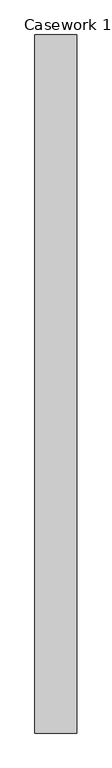
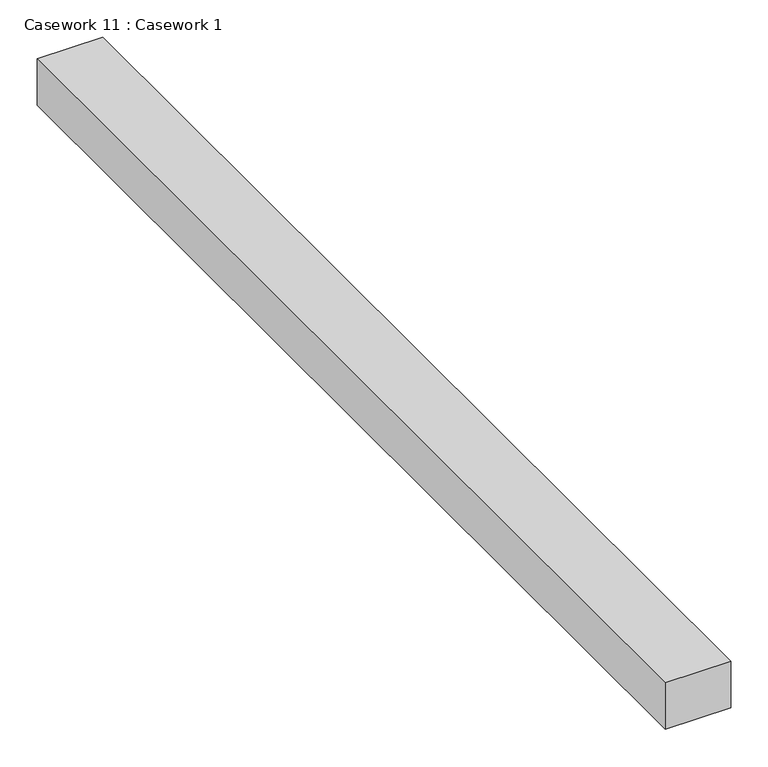
"""IFC4 building model written with IfcOpenShell, lengths in millimetres: furniture geometry, Casework 11 : Casework 1."""

from ifc_helpers import new_model, si_unit, frame, origin, place, context, project, spatial, polyline, outline, extrude, source, transform, mapped, element, save


def casework_11_casework_1_2f257332(model_context):
    return source(origin(), model_context, "Body", "SweptSolid", [
        extrude(outline(polyline([(6614.5559589, 14787.9496924), (6614.5559589, 13098.8496924), (6512.9559589, 13098.8496924), (6512.9559589, 14787.9496924), (6614.5559589, 14787.9496924)])), frame((0.0, 0.0, 3581.4), z_axis=(0.0, 0.0, 1.0), x_axis=(1.0, 0.0, 0.0)), (0.0, 0.0, 1.0), 76.2),
    ])


if __name__ == "__main__":
    model = new_model("IFC4")
    model_context = context("Model", 3, world=origin())
    ifc_project = project(units=[si_unit("LENGTHUNIT", "METRE", prefix="MILLI")], contexts=[model_context])
    site = spatial("IfcSite", under=ifc_project)
    building = spatial("IfcBuilding", under=site)
    placement = place(None, origin())
    casework_11_casework_1_shape = casework_11_casework_1_2f257332(model_context)
    element("IfcFurniture", 1, ObjectType="Casework 11 : Casework 1", at=placement, inside=building, context=model_context, shape_type="MappedRepresentation", body=[
        mapped(casework_11_casework_1_shape, transform((0.0, 0.0, 0.0), x_axis=(1.0, 0.0, 0.0), y_axis=(0.0, 1.0, 0.0), z_axis=(0.0, 0.0, 1.0))),
    ])
    save(model, "model.ifc")

# Revit data of these elements
# Element 1 (IfcFurniture, "Casework 11 : Casework 1")
#   Materials on its faces: "Clad - White"
# Materials
#   "Clad - White": class "Wood", colour RGB 242 242 238, transparency 0, Cost = 0
